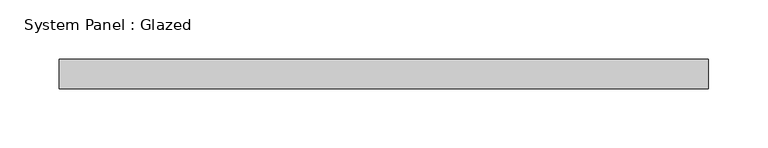
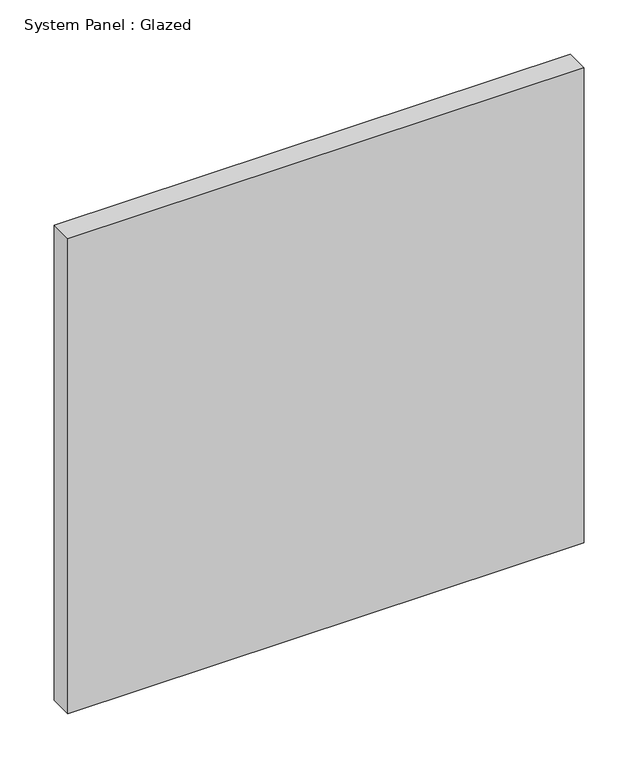
"""IFC4 building model written with IfcOpenShell, lengths in millimetres: plate geometry, System Panel : Glazed."""

from ifc_helpers import new_model, si_unit, origin, origin_with_axes, place, context, project, spatial, polyline, outline, extrude, source, transform, mapped, element, save


def system_panel_glazed_ea2acdbe(model_context):
    return source(origin(), model_context, "Body", "SweptSolid", [
        extrude(outline(polyline([(275.0, 24.5), (-275.0, 24.5), (-275.0, 49.5), (275.0, 49.5), (275.0, 24.5)])), origin_with_axes(), (0.0, 0.0, 1.0), 535.0),
    ])


if __name__ == "__main__":
    model = new_model("IFC4")
    model_context = context("Model", 3, world=origin())
    ifc_project = project(units=[si_unit("LENGTHUNIT", "METRE", prefix="MILLI")], contexts=[model_context])
    site = spatial("IfcSite", under=ifc_project)
    building = spatial("IfcBuilding", under=site)
    placement = place(None, origin())
    system_panel_glazed_shape = system_panel_glazed_ea2acdbe(model_context)
    element("IfcPlate", 1, ObjectType="System Panel : Glazed", at=placement, inside=building, context=model_context, shape_type="MappedRepresentation", body=[
        mapped(system_panel_glazed_shape, transform((0.0, 0.0, 0.0), x_axis=(1.0, 0.0, 0.0), y_axis=(0.0, 1.0, 0.0), z_axis=(0.0, 0.0, 1.0))),
    ])
    save(model, "model.ifc")

# Revit data of these elements
# Type "System Panel : Glazed"
#   Construction Type Id = "GSP4R"
#   Analytic Construction = "1/8 in Pilkington single glazing"
#   Visual Light Transmittance = 0.9
#   Solar Heat Gain Coefficient = 0.86
#   Heat Transfer Coefficient (U) = 6.7069 W/(m²·K)
#   Define Thermal Properties by = 1
# Element 1 (IfcPlate, "System Panel : Glazed")
#   Materials on its faces: "Glass"
# Materials
#   "Glass": class "Glass", colour RGB 0 128 192, transparency 0.9, Description = "Soda Lime Glass", Cost = 0
